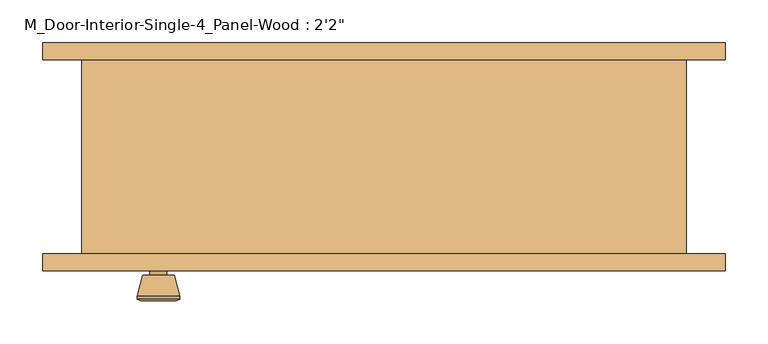
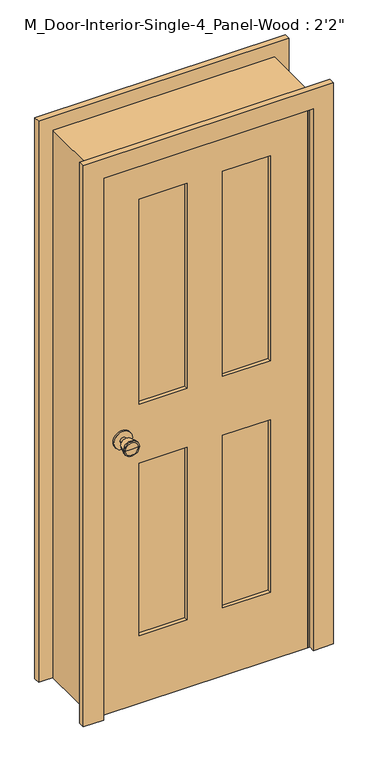
"""IFC4 building model written with IfcOpenShell, lengths in millimetres: door geometry."""

from ifc_helpers import new_model, si_unit, point, frame, frame_2d, origin, place, context, project, spatial, polyline, circle_curve, trimmed, segment, composite_curve, outline, extrude, faceted_brep, source, transform, mapped, element, save
from ifc_brep_helpers import plane_surface, cylinder_surface, revolved_surface, advanced_brep


def door_a34dad57(model_context):
    return source(origin(), model_context, "Body", "SolidModel", [
        advanced_brep(
        [(-265.2, -70.125, 914.4), (-275.2, -70.125, 914.4), (-255.2, -70.125, 914.4), (-244.7241324, -21.125, 914.4), (-285.6758676, -21.125, 914.4), (-265.2, -21.125, 914.4), (-240.2, -22.9528681, 914.4), (-290.2, -22.9528681, 914.4), (-240.2, -26.4165463, 914.4), (-290.2, -26.4165463, 914.4), (-246.563764, -51.125, 914.4), (-283.836236, -51.125, 914.4), (-255.2, -51.125, 914.4), (-275.2, -51.125, 914.4)],
        [
            (0, 1),
            (1, 2, circle_curve(frame((-265.2, -70.125, 914.4), z_axis=(0.0, -1.0, 0.0), x_axis=(-1.0, 0.0, 0.0)), 10.0)),
            (2, 0),
            (2, 1, circle_curve(frame((-265.2, -70.125, 914.4), z_axis=(0.0, -1.0, 0.0), x_axis=(-1.0, 0.0, 0.0)), 10.0)),
            (3, 4, circle_curve(frame((-265.2, -21.125, 914.4), z_axis=(0.0, 1.0, 0.0), x_axis=(-1.0, 0.0, 0.0)), 20.4758676)),
            (4, 5),
            (5, 3),
            (4, 3, circle_curve(frame((-265.2, -21.125, 914.4), z_axis=(0.0, 1.0, 0.0), x_axis=(-1.0, 0.0, 0.0)), 20.4758676)),
            (6, 7, circle_curve(frame((-265.2, -22.9528681, 914.4), z_axis=(0.0, 1.0, 0.0), x_axis=(-1.0, 0.0, 0.0)), 25.0)),
            (7, 4),
            (3, 6),
            (7, 6, circle_curve(frame((-265.2, -22.9528681, 914.4), z_axis=(0.0, 1.0, 0.0), x_axis=(-1.0, 0.0, 0.0)), 25.0)),
            (8, 9, circle_curve(frame((-265.2, -26.4165463, 914.4), z_axis=(0.0, 1.0, 0.0), x_axis=(-1.0, 0.0, 0.0)), 25.0)),
            (9, 7),
            (6, 8),
            (9, 8, circle_curve(frame((-265.2, -26.4165463, 914.4), z_axis=(0.0, 1.0, 0.0), x_axis=(-1.0, 0.0, 0.0)), 25.0)),
            (10, 11, circle_curve(frame((-265.2, -51.125, 914.4), z_axis=(0.0, 1.0, 0.0), x_axis=(-1.0, 0.0, 0.0)), 18.636236)),
            (11, 9),
            (8, 10),
            (11, 10, circle_curve(frame((-265.2, -51.125, 914.4), z_axis=(0.0, 1.0, 0.0), x_axis=(-1.0, 0.0, 0.0)), 18.636236)),
            (12, 13, circle_curve(frame((-265.2, -51.125, 914.4), z_axis=(0.0, 1.0, 0.0), x_axis=(-1.0, 0.0, 0.0)), 10.0)),
            (13, 11),
            (10, 12),
            (13, 12, circle_curve(frame((-265.2, -51.125, 914.4), z_axis=(0.0, 1.0, 0.0), x_axis=(-1.0, 0.0, 0.0)), 10.0)),
            (1, 13),
            (12, 2),
        ],
        [
            plane_surface(frame((-265.2, -70.125, 914.4), z_axis=(0.0, -1.0, 0.0), x_axis=(-1.0, 0.0, 0.0))),
            plane_surface(frame((-265.2, -21.125, 914.4), z_axis=(0.0, 1.0, 0.0), x_axis=(-1.0, 0.0, 0.0))),
            revolved_surface(polyline([(-285.6758676, -21.125, 914.4), (-290.2, -22.9528681, 914.4)]), (-265.2, -70.125, 914.4), (0.0, -1.0, 0.0)),
            cylinder_surface(frame((-265.2, -70.125, 914.4), z_axis=(0.0, -1.0, 0.0), x_axis=(-1.0, 0.0, 0.0)), 25.0),
            revolved_surface(polyline([(-290.2, -26.4165463, 914.4), (-283.836236, -51.125, 914.4)]), (-265.2, -70.125, 914.4), (0.0, -1.0, 0.0)),
            plane_surface(frame((-265.2, -51.125, 914.4), z_axis=(0.0, -1.0, 0.0), x_axis=(-1.0, 0.0, 0.0))),
            cylinder_surface(frame((-265.2, -70.125, 914.4), z_axis=(0.0, -1.0, 0.0), x_axis=(-1.0, 0.0, 0.0)), 10.0),
        ],
        [
            (0, [[1, 2, 3]]),
            (0, [[-3, 4, -1]]),
            (1, [[5, 6, 7]]),
            (1, [[8, -7, -6]]),
            (2, [[9, 10, -5, 11]]),
            (2, [[12, -11, -8, -10]]),
            (3, [[13, 14, -9, 15]]),
            (3, [[16, -15, -12, -14]]),
            (4, [[17, 18, -13, 19]]),
            (4, [[20, -19, -16, -18]]),
            (5, [[21, 22, -17, 23]]),
            (5, [[24, -23, -20, -22]]),
            (6, [[-2, 25, -21, 26]]),
            (6, [[-4, -26, -24, -25]]),
        ],
    ),
        extrude(outline(composite_curve([segment(trimmed(circle_curve(frame_2d((914.4, -265.2)), 30.0), [point((914.4, -295.2))], [point((914.4, -235.2))], False, "CARTESIAN"), True, "CONTINUOUS"), segment(trimmed(circle_curve(frame_2d((914.4, -265.2)), 30.0), [point((914.4, -235.2))], [point((914.4, -295.2))], False, "CARTESIAN"), True, "CONTINUOUS")], self_intersect=False)), frame((0.0, -76.125, 0.0), z_axis=(0.0, 1.0, 0.0), x_axis=(0.0, 0.0, 1.0)), (0.0, 0.0, 1.0), 6.0),
        advanced_brep(
        [(-265.2, -117.125, 914.4), (-255.2, -117.125, 914.4), (-275.2, -117.125, 914.4), (-244.7241324, -166.125, 914.4), (-265.2, -166.125, 914.4), (-285.6758676, -166.125, 914.4), (-240.2, -164.2971319, 914.4), (-290.2, -164.2971319, 914.4), (-240.2, -160.8334537, 914.4), (-290.2, -160.8334537, 914.4), (-246.563764, -136.125, 914.4), (-283.836236, -136.125, 914.4), (-255.2, -136.125, 914.4), (-275.2, -136.125, 914.4)],
        [
            (0, 1),
            (1, 2, circle_curve(frame((-265.2, -117.125, 914.4), z_axis=(0.0, 1.0, 0.0), x_axis=(-1.0, 0.0, 0.0)), 10.0)),
            (2, 0),
            (2, 1, circle_curve(frame((-265.2, -117.125, 914.4), z_axis=(0.0, 1.0, 0.0), x_axis=(-1.0, 0.0, 0.0)), 10.0)),
            (3, 4),
            (4, 5),
            (5, 3, circle_curve(frame((-265.2, -166.125, 914.4), z_axis=(0.0, -1.0, 0.0), x_axis=(-1.0, 0.0, 0.0)), 20.4758676)),
            (3, 5, circle_curve(frame((-265.2, -166.125, 914.4), z_axis=(0.0, -1.0, 0.0), x_axis=(-1.0, 0.0, 0.0)), 20.4758676)),
            (6, 3),
            (5, 7),
            (7, 6, circle_curve(frame((-265.2, -164.2971319, 914.4), z_axis=(0.0, -1.0, 0.0), x_axis=(-1.0, 0.0, 0.0)), 25.0)),
            (6, 7, circle_curve(frame((-265.2, -164.2971319, 914.4), z_axis=(0.0, -1.0, 0.0), x_axis=(-1.0, 0.0, 0.0)), 25.0)),
            (8, 6),
            (7, 9),
            (9, 8, circle_curve(frame((-265.2, -160.8334537, 914.4), z_axis=(0.0, -1.0, 0.0), x_axis=(-1.0, 0.0, 0.0)), 25.0)),
            (8, 9, circle_curve(frame((-265.2, -160.8334537, 914.4), z_axis=(0.0, -1.0, 0.0), x_axis=(-1.0, 0.0, 0.0)), 25.0)),
            (10, 8),
            (9, 11),
            (11, 10, circle_curve(frame((-265.2, -136.125, 914.4), z_axis=(0.0, -1.0, 0.0), x_axis=(-1.0, 0.0, 0.0)), 18.636236)),
            (10, 11, circle_curve(frame((-265.2, -136.125, 914.4), z_axis=(0.0, -1.0, 0.0), x_axis=(-1.0, 0.0, 0.0)), 18.636236)),
            (12, 10),
            (11, 13),
            (13, 12, circle_curve(frame((-265.2, -136.125, 914.4), z_axis=(0.0, -1.0, 0.0), x_axis=(-1.0, 0.0, 0.0)), 10.0)),
            (12, 13, circle_curve(frame((-265.2, -136.125, 914.4), z_axis=(0.0, -1.0, 0.0), x_axis=(-1.0, 0.0, 0.0)), 10.0)),
            (1, 12),
            (13, 2),
        ],
        [
            plane_surface(frame((-265.2, -117.125, 914.4), z_axis=(0.0, 1.0, 0.0), x_axis=(-1.0, 0.0, 0.0))),
            plane_surface(frame((-265.2, -166.125, 914.4), z_axis=(0.0, -1.0, 0.0), x_axis=(-1.0, 0.0, 0.0))),
            revolved_surface(polyline([(-285.6758676, -166.125, 914.4), (-290.2, -164.2971319, 914.4)]), (-265.2, -117.125, 914.4), (0.0, 1.0, 0.0)),
            cylinder_surface(frame((-265.2, -117.125, 914.4), z_axis=(0.0, 1.0, 0.0), x_axis=(-1.0, 0.0, 0.0)), 25.0),
            revolved_surface(polyline([(-290.2, -160.8334537, 914.4), (-283.836236, -136.125, 914.4)]), (-265.2, -117.125, 914.4), (0.0, 1.0, 0.0)),
            plane_surface(frame((-265.2, -136.125, 914.4), z_axis=(0.0, 1.0, 0.0), x_axis=(-1.0, 0.0, 0.0))),
            cylinder_surface(frame((-265.2, -117.125, 914.4), z_axis=(0.0, 1.0, 0.0), x_axis=(-1.0, 0.0, 0.0)), 10.0),
        ],
        [
            (0, [[1, 2, 3]]),
            (0, [[-3, 4, -1]]),
            (1, [[5, 6, 7]]),
            (1, [[-6, -5, 8]]),
            (2, [[9, -7, 10, 11]]),
            (2, [[-10, -8, -9, 12]]),
            (3, [[13, -11, 14, 15]]),
            (3, [[-14, -12, -13, 16]]),
            (4, [[17, -15, 18, 19]]),
            (4, [[-18, -16, -17, 20]]),
            (5, [[21, -19, 22, 23]]),
            (5, [[-22, -20, -21, 24]]),
            (6, [[25, -23, 26, -2]]),
            (6, [[-26, -24, -25, -4]]),
        ],
    ),
        extrude(outline(composite_curve([segment(trimmed(circle_curve(frame_2d((914.4, -265.2)), 30.0), [point((914.4, -295.2))], [point((914.4, -235.2))], False, "CARTESIAN"), True, "CONTINUOUS"), segment(trimmed(circle_curve(frame_2d((914.4, -265.2)), 30.0), [point((914.4, -235.2))], [point((914.4, -295.2))], False, "CARTESIAN"), True, "CONTINUOUS")], self_intersect=False)), frame((0.0, -117.125, 0.0), z_axis=(0.0, 1.0, 0.0), x_axis=(0.0, 0.0, 1.0)), (0.0, 0.0, 1.0), 6.0),
        faceted_brep([(355.2, -111.125, 0.0), (330.2, -111.125, 0.0), (330.2, -76.125, 0.0), (317.5, -76.125, 0.0), (317.5, -41.2, 0.0), (330.2, -41.2, 0.0), (330.2, 117.475, 0.0), (355.2, 117.475, 0.0), (355.2, 117.475, 1853.8), (355.2, -111.125, 1853.8), (330.2, 117.475, 1828.8), (-330.2, 117.475, 1828.8), (-330.2, 117.475, 0.0), (-355.2, 117.475, 0.0), (-355.2, 117.475, 1853.8), (330.2, -41.2, 1828.8), (317.5, -41.2, 1816.1), (-317.5, -41.2, 1816.1), (-317.5, -41.2, 0.0), (-330.2, -41.2, 0.0), (-330.2, -41.2, 1828.8), (317.5, -76.125, 1816.1), (330.2, -76.125, 1828.8), (-330.2, -76.125, 1828.8), (-330.2, -76.125, 0.0), (-317.5, -76.125, 0.0), (-317.5, -76.125, 1816.1), (330.2, -111.125, 1828.8), (-355.2, -111.125, 1853.8), (-355.2, -111.125, 0.0), (-330.2, -111.125, 0.0), (-330.2, -111.125, 1828.8)], [[[0, 1, 2, 3, 4, 5, 6, 7]], [[7, 8, 9, 0]], [[6, 10, 11, 12, 13, 14, 8, 7]], [[5, 15, 10, 6]], [[4, 16, 17, 18, 19, 20, 15, 5]], [[3, 21, 16, 4]], [[2, 22, 23, 24, 25, 26, 21, 3]], [[1, 27, 22, 2]], [[0, 9, 28, 29, 30, 31, 27, 1]], [[8, 14, 28, 9]], [[15, 20, 11, 10]], [[21, 26, 17, 16]], [[27, 31, 23, 22]], [[29, 13, 12, 19, 18, 25, 24, 30]], [[14, 13, 29, 28]], [[20, 19, 12, 11]], [[26, 25, 18, 17]], [[31, 30, 24, 23]]]),
        extrude(outline(polyline([(1828.8, -330.2), (0.0, -330.2), (0.0, 330.2), (1828.8, 330.2), (1828.8, -330.2)]), holes=[polyline([(1708.8, 57.5), (1708.8, 210.2), (1014.4, 210.2), (1014.4, 57.5), (1708.8, 57.5)]), polyline([(1014.4, -57.5), (1014.4, -210.2), (1708.8, -210.2), (1708.8, -57.5), (1014.4, -57.5)]), polyline([(814.4, 57.5), (814.4, 210.2), (230.0, 210.2), (230.0, 57.5), (814.4, 57.5)]), polyline([(230.0, -57.5), (230.0, -210.2), (814.4, -210.2), (814.4, -57.5), (230.0, -57.5)])]), frame((0.0, -111.125, 0.0), z_axis=(0.0, 1.0, 0.0), x_axis=(0.0, 0.0, 1.0)), (0.0, 0.0, 1.0), 35.0),
        extrude(outline(polyline([(210.2, -87.7916667), (210.2, -99.4583333), (57.5, -99.4583333), (57.5, -87.7916667), (210.2, -87.7916667)])), frame((0.0, 0.0, 1014.4), z_axis=(0.0, 0.0, 1.0), x_axis=(1.0, 0.0, 0.0)), (0.0, 0.0, 1.0), 694.4),
        extrude(outline(polyline([(-57.5, -87.7916667), (-57.5, -99.4583333), (-210.2, -99.4583333), (-210.2, -87.7916667), (-57.5, -87.7916667)])), frame((0.0, 0.0, 1014.4), z_axis=(0.0, 0.0, 1.0), x_axis=(1.0, 0.0, 0.0)), (0.0, 0.0, 1.0), 694.4),
        extrude(outline(polyline([(210.2, -87.7916667), (210.2, -99.4583333), (57.5, -99.4583333), (57.5, -87.7916667), (210.2, -87.7916667)])), frame((0.0, 0.0, 230.0), z_axis=(0.0, 0.0, 1.0), x_axis=(1.0, 0.0, 0.0)), (0.0, 0.0, 1.0), 584.4),
        extrude(outline(polyline([(-57.5, -87.7916667), (-57.5, -99.4583333), (-210.2, -99.4583333), (-210.2, -87.7916667), (-57.5, -87.7916667)])), frame((0.0, 0.0, 230.0), z_axis=(0.0, 0.0, 1.0), x_axis=(1.0, 0.0, 0.0)), (0.0, 0.0, 1.0), 584.4),
        extrude(outline(polyline([(0.0, 401.55), (1900.15, 401.55), (1900.15, -401.55), (0.0, -401.55), (0.0, -336.55), (1835.15, -336.55), (1835.15, 336.55), (0.0, 336.55), (0.0, 401.55)])), frame((0.0, -131.125, 0.0), z_axis=(0.0, 1.0, 0.0), x_axis=(0.0, 0.0, 1.0)), (0.0, 0.0, 1.0), 20.0),
        extrude(outline(polyline([(0.0, 401.55), (1900.15, 401.55), (1900.15, -401.55), (0.0, -401.55), (0.0, -336.55), (1835.15, -336.55), (1835.15, 336.55), (0.0, 336.55), (0.0, 401.55)])), frame((0.0, 117.475, 0.0), z_axis=(0.0, 1.0, 0.0), x_axis=(0.0, 0.0, 1.0)), (0.0, 0.0, 1.0), 20.0),
    ])


if __name__ == "__main__":
    model = new_model("IFC4")
    model_context = context("Model", 3, world=origin())
    ifc_project = project(units=[si_unit("LENGTHUNIT", "METRE", prefix="MILLI")], contexts=[model_context])
    site = spatial("IfcSite", under=ifc_project)
    building = spatial("IfcBuilding", under=site)
    placement = place(None, origin())
    door_shape = door_a34dad57(model_context)
    element("IfcDoor", 1, ObjectType="M_Door-Interior-Single-4_Panel-Wood : 2'2\"", at=placement, inside=building, context=model_context, shape_type="MappedRepresentation", body=[
        mapped(door_shape, transform((0.0, 0.0, 0.0), x_axis=(1.0, 0.0, 0.0), y_axis=(0.0, 1.0, 0.0), z_axis=(0.0, 0.0, 1.0))),
    ])
    save(model, "model.ifc")

# Revit data of these elements
# Type "M_Door-Interior-Single-4_Panel-Wood : 2'2\""
#   Type Mark = "43"
#   Assembly Code = "C1020300"
#   Analytic Construction = "Wooden"
#   Top Rail = 0' - 4.72441"
#   Thickness = 0' - 1.37795"
#   Thermal Resistance (R) = 0.455703 (m²·K)/W
#   Swing Angle [instance default] = 90.00°
#   Stiles = 0' - 4.72441"
#   Rough Width = 2' - 3.9685"
#   Rough Height = 6' - 0.98425"
#   Mullion = 0' - 4.52756"
#   Lock Rail = 0' - 7.87402"
#   Height = 6' - 0"
#   Width = 2' - 2"
#   Heat Transfer Coefficient (U) = 2.19465 W/(m²·K)
#   Bottom Rail = 0' - 9.05512"
#   Trim Material = Cherry
#   Panel Material = Cherry
#   Frame Material = Cherry
#   Door Handle Material = Aluminum
#   Visual Light Transmittance = 0
#   Solar Heat Gain Coefficient = 0
#   Wall Closure = (empty or 0)
#   Function = (empty or 0)
# Element 1 (IfcDoor, "M_Door-Interior-Single-4_Panel-Wood : 2'2\"")
#   Materials on its faces: "Cherry", "Aluminum"
# Materials
#   "Cherry": class "Wood", colour RGB 226 177 128, transparency 0, Description = "Prunus Serotina", Cost = 0
#   "Aluminum": class "Metal", colour RGB 247 247 247, transparency 0, Description = "Aluminum 6061", Cost = 0
